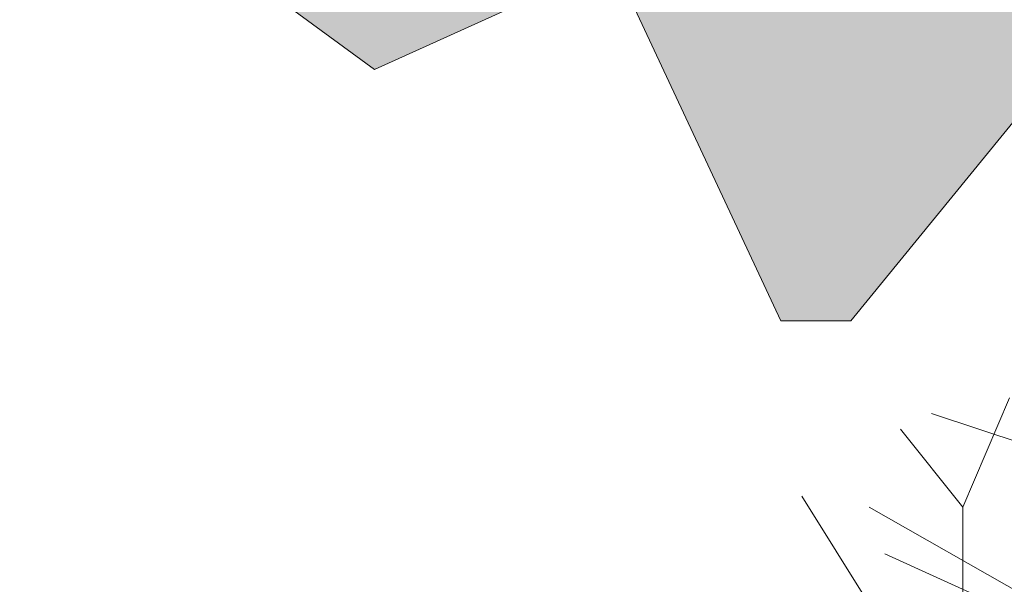
# Model space of a CAD drawing. Units: inches. Extents: x 2091 to 2899, y 967 to 2217.
# Tile 105 of 256: x 2223 to 2254, y 1114 to 1131. Entities that reach past the tile are written whole.
import ezdxf

# ---------------------------------------------------------------- set-up
doc = ezdxf.new("R2010")
doc.units = ezdxf.units.IN
doc.layers.add('A-ANNO-DIMS', color=2, linetype='Continuous', lineweight=18)
doc.layers.add('L-PLNT-TREE', color=94, linetype='Continuous', lineweight=13)
doc.layers.add('A-WALL-PATT', color=141, linetype='Continuous', lineweight=13, true_color=0xadddf7)
doc.layers.add('L-PLNT-PATT', color=114, linetype='Continuous', lineweight=13, true_color=0x139b48)
doc.styles.get("Standard").update_dxf_attribs({"font": 'arial.ttf'})
doc.dimstyles.new('ISO-25', dxfattribs={"dimtxt": 4, "dimasz": 4, "dimexe": 1.25, "dimexo": 0.625, "dimtad": 1, "dimdec": 0, "dimlunit": 3, "dimtxsty": 'Standard', "dimcen": 2.5, "dimadec": 0, "dimazin": 0, "dimtfac": 1, "dimtdec": 0, "dimtmove": 0, "dimatfit": 3, "dimfxl": 1, "dimarcsym": 0})

# ---------------------------------------------------------------- blocks, each defined once
blk = doc.blocks.new('*U25')
blk.add_lwpolyline([(-1139.42368, 1783.79628), (-1216.11644, 1685.47796), (-1117.5111, 1601.2033), (-1051.7759, 1643.3419), (-1126.09884, 1521.20092), (-1072.10606, 1527.49758), (-1079.90386, 1416.93646), (-1259.93906, 1179.83508), (-1479.05978, 1165.78888), (-1577.66258, 1109.60662), (-1742.00312, 927.01364), (-1676.26538, 814.64658), (-1270.89408, 828.69278), (-1194.20386, 772.51052), (-1007.95074, 856.78518), (-876.4778, 575.87134), (-821.70016, 575.87134), (-569.71184, 884.87504)])
blk = doc.blocks.new('*U29')
for p, q in [((-426.72, 414.528), (-390.144, 499.872)), ((-377.952, 463.296), (-451.104, 487.68)), ((-426.72, 414.528), (-475.488, 475.488)), ((-463.296, 280.416), (-552.577, 423.037)), ((-329.184, 316.992), (-499.872, 414.528)), ((-426.72, 316.992), (-426.72, 414.528)), ((-353.568, 316.992), (-487.68, 377.952))]:
    blk.add_line(p, q)
blk = doc.blocks.new('*D71')
at = {"layer": 'A-ANNO-DIMS', "color": 0, "lineweight": -2, "transparency": 16777216}
for p, q in [((2212.144, 1351.294), (2212.144, 969.464)), ((2452.144, 1351.294), (2452.144, 969.464)), ((2216.144, 970.714), (2448.144, 970.714))]:
    blk.add_line(p, q, dxfattribs=at)
at = {"layer": 'A-ANNO-DIMS', "color": 0, "transparency": 16777216}
for points in [[(2216.144, 971.381), (2216.144, 970.048), (2212.144, 970.714)], [(2448.144, 971.381), (2448.144, 970.048), (2452.144, 970.714)]]:
    blk.add_solid(points, dxfattribs=at)
at = {"layer": 'Defpoints', "color": 0, "transparency": 16777216}
for p in [(2212.144, 1351.919), (2452.144, 1351.919), (2452.144, 970.714)]:
    blk.add_point(p, dxfattribs=at)
at = {"layer": 'A-ANNO-DIMS', "color": 0, "transparency": 16777216, "insert": (2332.144, 973.382), "char_height": 4, "attachment_point": 5}
blk.add_mtext('20\'-0"', dxfattribs=at)
blk = doc.blocks.new('*D75')
at = {"layer": 'A-ANNO-DIMS', "color": 0, "lineweight": -2, "transparency": 16777216}
for p, q in [((2212.144, 1274.794), (2212.144, 969.464)), ((2308.144, 1274.794), (2308.144, 969.464)), ((2216.144, 970.714), (2304.144, 970.714))]:
    blk.add_line(p, q, dxfattribs=at)
at = {"layer": 'A-ANNO-DIMS', "color": 0, "transparency": 16777216}
for points in [[(2216.144, 971.381), (2216.144, 970.048), (2212.144, 970.714)], [(2304.144, 971.381), (2304.144, 970.048), (2308.144, 970.714)]]:
    blk.add_solid(points, dxfattribs=at)
at = {"layer": 'Defpoints', "color": 0, "transparency": 16777216}
for p in [(2212.144, 1275.419), (2308.144, 1275.419), (2308.144, 970.714)]:
    blk.add_point(p, dxfattribs=at)
at = {"layer": 'A-ANNO-DIMS', "color": 0, "transparency": 16777216, "insert": (2260.144, 973.382), "char_height": 4, "attachment_point": 5}
blk.add_mtext('8\'-0"', dxfattribs=at)

msp = doc.modelspace()

# ---------------------------------------------------------------- hatches: boundary and pattern name
at = {"layer": 'A-WALL-PATT'}
h = msp.add_hatch(color=256, dxfattribs=at)
h.dxf.hatch_style = 1
h.paths.add_polyline_path([(2803.144, 2050.919), (2203.144, 2050.919), (2203.144, 1090.919), (2803.144, 1090.919)])
h.paths.add_polyline_path([(2635.799, 1147.54), (2674.524, 1147.54, 0.376086), (2678.53, 1152.88), (2678.53, 1159.556, 0.333335), (2674.524, 1163.562), (2674.524, 1163.562), (2674.524, 1192.934), (2635.806, 1192.934), (2597.088, 1192.934), (2597.088, 1163.562, 0.333335), (2593.082, 1159.556), (2593.082, 1152.88, 0.376086), (2597.088, 1147.54)], flags=0)
h.paths.add_polyline_path([(2436.01, 1278.241, 0.000483), (2435.953, 1278.215, -0.001328), (2435.936, 1278.112, -0.001711), (2436.116, 1278.041, 0.002185)], flags=0)
h.paths.add_polyline_path([(2794.144, 1143.419), (2794.144, 1347.419), (2543.37, 1347.419), (2543.37, 1351.919), (2794.144, 1351.919), (2794.144, 1392.714), (2793.947, 1392.714), (2793.947, 1473.537), (2794.144, 1473.537), (2794.144, 1531.919), (2650.144, 1531.919), (2650.144, 1536.419), (2794.144, 1536.419), (2794.144, 1692.419), (2609.376, 1692.419), (2609.376, 1644.419), (2604.876, 1644.419), (2604.876, 1744.919), (2609.376, 1744.919), (2609.376, 1696.919), (2794.144, 1696.919), (2794.144, 1780.919), (2609.644, 1780.919), (2493.876, 1780.919), (2493.876, 1785.419), (2609.644, 1785.419), (2794.144, 1785.419), (2794.144, 1847.939), (2793.951, 1847.939), (2793.951, 1928.762), (2794.144, 1928.762), (2794.144, 1941.419), (2614.144, 1941.419), (2614.144, 1821.419), (2609.644, 1821.419), (2609.644, 1941.419), (2392.144, 1941.419), (2392.144, 1819.919), (2387.644, 1819.919), (2387.644, 1941.419), (2212.144, 1941.419), (2212.144, 1783.919), (2392.144, 1783.919), (2392.144, 1780.919), (2212.144, 1780.919), (2212.144, 1629.419), (2387.644, 1629.419), (2387.644, 1744.919), (2392.144, 1744.919), (2392.144, 1627.919), (2317.144, 1627.919), (2317.144, 1551.419), (2317.144, 1536.419), (2459.384, 1536.419), (2459.384, 1602.396), (2463.884, 1602.396), (2463.884, 1531.919), (2456.644, 1531.919), (2456.644, 1529.919), (2452.144, 1529.919), (2452.144, 1531.919), (2312.644, 1531.919), (2312.644, 1551.419), (2306.144, 1551.419), (2306.144, 1555.919), (2308.144, 1555.919), (2308.144, 1551.419), (2312.644, 1551.419), (2312.644, 1627.919), (2212.144, 1627.919), (2212.144, 1555.919), (2270.144, 1555.919), (2270.144, 1551.419), (2212.144, 1551.419), (2212.144, 1351.919), (2272.144, 1351.919), (2272.144, 1347.419), (2212.144, 1347.419), (2212.144, 1275.419), (2308.144, 1275.419), (2308.144, 1351.919), (2452.144, 1351.919), (2452.144, 1493.919), (2456.644, 1493.919), (2456.644, 1347.419), (2312.644, 1347.419), (2312.644, 1270.919), (2212.144, 1270.919), (2212.144, 1099.919), (2281.238, 1099.919), (2282.871, 1110.914), (2282.008, 1116.997), (2278.558, 1121.42), (2268.206, 1128.056), (2272.088, 1128.056), (2273.813, 1131.927), (2279.42, 1134.692), (2285.028, 1135.245), (2287.616, 1137.457), (2288.047, 1138.01), (2289.341, 1140.775), (2291.067, 1139.669), (2292.361, 1135.245), (2295.38, 1136.904), (2296.243, 1135.798), (2297.105, 1133.033), (2300.125, 1138.01), (2303.144, 1138.01), (2304.438, 1135.798), (2303.144, 1133.586), (2306.595, 1134.692), (2307.889, 1133.033), (2310.908, 1135.245), (2313.927, 1134.139), (2315.627, 1132.427), (2308.32, 1117.55), (2290.204, 1109.808), (2288.91, 1103.172), (2289.272, 1099.919), (2434.918, 1099.919), (2431.593, 1124.788), (2429.93, 1169.553), (2430.927, 1240.52), (2435.659, 1238.186), (2437.135, 1196.554), (2438.798, 1143.973), (2442.678, 1111.998), (2446.558, 1099.919), (2794.144, 1099.919), (2794.144, 1138.919), (2548.032, 1138.919), (2548.032, 1143.419), (2548.032, 1148.819), (2546.668, 1148.032), (2528.686, 1179.179, 0.256256), (2512.032, 1148.819), (2512.032, 1143.419), (2512.032, 1138.919), (2507.532, 1138.919), (2507.532, 1143.419), (2507.532, 1148.819, 0.256256), (2490.879, 1179.179), (2472.896, 1148.032), (2471.532, 1148.819), (2471.532, 1143.419), (2467.032, 1143.419), (2467.032, 1269.946, 0.039061), (2460.91, 1273.58), (2467.032, 1273.58), (2467.032, 1286.325, 0.014511), (2465.216, 1286.762), (2467.032, 1287.053), (2467.032, 1323.419), (2471.532, 1323.419), (2471.532, 1148.819), (2489.532, 1179.996), (2490.896, 1179.208), (2490.879, 1179.179, -0.256256), (2507.532, 1148.819), (2507.532, 1143.419), (2512.032, 1143.419), (2512.032, 1148.819, -0.256256), (2528.686, 1179.179), (2528.668, 1179.208), (2530.032, 1179.996), (2548.032, 1148.819), (2548.032, 1143.419)], flags=16)
h.paths.add_polyline_path([(2607.769, 1200.945), (2607.769, 1265.031), (2597.088, 1281.052), (2619.785, 1281.052), (2627.795, 1337.127), (2635.799, 1337.127), (2643.817, 1337.127), (2651.827, 1281.052), (2674.524, 1281.052), (2663.843, 1265.031), (2663.843, 1200.945), (2635.806, 1200.945)], flags=0)
edge = h.paths.add_edge_path(flags=0)
edge.add_ellipse((13303.896, 1272.999), major_axis=(-10595.313, 0), ratio=0.84230387, start_angle=0.6282372, end_angle=0.6465541, ccw=False)
edge.add_ellipse((2711.7, 1156.853), major_axis=(2.22, 0), ratio=0.842304, start_angle=111.5352, end_angle=180.6282, ccw=False)
edge.add_ellipse((13303.156, 1272.999), major_axis=(-10593.026, 0), ratio=0.84230387, start_angle=0.5282715, end_angle=0.6465541, ccw=False)
edge.add_line((2710.765, 1175.333), (2710.13, 1175.333))
edge.add_ellipse((2710.13, 1176.58), major_axis=(1.48, 0), ratio=0.842304, start_angle=180, end_angle=270, ccw=False)
edge.add_line((2708.65, 1176.58), (2708.65, 1200.783))
edge.add_ellipse((2710.13, 1200.783), major_axis=(1.48, 0), ratio=0.842304, start_angle=90, end_angle=180, ccw=False)
edge.add_line((2710.13, 1202.029), (2710.465, 1202.029))
edge.add_ellipse((13303.156, 1272.999), major_axis=(-10593.026, 0), ratio=0.84230387, start_angle=-0.0902291, end_angle=0.3838668, ccw=False)
edge.add_ellipse((2710.13, 1290.927), major_axis=(-1.48, 0), ratio=0.842304, start_angle=0, end_angle=90, ccw=False)
edge.add_line((2708.65, 1290.927), (2708.65, 1315.13))
edge.add_ellipse((2710.13, 1315.13), major_axis=(-1.48, 0), ratio=0.842304, start_angle=-90, end_angle=0, ccw=False)
edge.add_line((2710.13, 1316.377), (2710.706, 1316.377))
edge.add_ellipse((3238.402, 1296.29), major_axis=(528.234, 0), ratio=0.8423039, start_angle=176.34957, end_angle=177.82005, ccw=False)
edge.add_ellipse((2775.063, 1071.451), major_axis=(313.308, 0), ratio=0.8423039, start_angle=102.12597, end_angle=103.78053, ccw=False)
edge.add_ellipse((2775.063, 1078.306), major_axis=(-305.303, 0), ratio=0.8423039, start_angle=-79.79046, end_angle=-77.55537, ccw=False)
edge.add_ellipse((2695.142, 1541.975), major_axis=(-250.96, 0), ratio=0.8423039, start_angle=99.25657, end_angle=102.55493)
edge.add_line((2741.41, 1334.214), (2747.133, 1337.378))
edge.add_ellipse((2747.539, 1336.857), major_axis=(-0.74, 0), ratio=0.842304, start_angle=270, end_angle=307.9331, ccw=False)
edge.add_ellipse((2747.539, 1336.857), major_axis=(-0.74, 0), ratio=0.842304, start_angle=232.0669, end_angle=270, ccw=False)
edge.add_line((2747.945, 1337.378), (2753.667, 1334.214))
edge.add_ellipse((2799.935, 1541.975), major_axis=(250.96, 0), ratio=0.8423039, start_angle=257.44507, end_angle=260.74343)
edge.add_ellipse((2720.014, 1078.306), major_axis=(305.303, 0), ratio=0.8423039, start_angle=77.55537, end_angle=79.79046, ccw=False)
edge.add_ellipse((2720.014, 1071.451), major_axis=(-313.308, 0), ratio=0.8423039, start_angle=256.21947, end_angle=257.87403, ccw=False)
edge.add_ellipse((2256.676, 1296.29), major_axis=(-528.234, 0), ratio=0.8423039, start_angle=182.17995, end_angle=183.65043, ccw=False)
edge.add_line((2784.371, 1316.377), (2784.947, 1316.377))
edge.add_ellipse((2784.947, 1315.13), major_axis=(1.48, 0), ratio=0.842304, start_angle=0, end_angle=90, ccw=False)
edge.add_line((2786.427, 1315.13), (2786.427, 1290.927))
edge.add_ellipse((2784.947, 1290.927), major_axis=(1.48, 0), ratio=0.842304, start_angle=270, end_angle=360, ccw=False)
edge.add_ellipse((-7808.079, 1272.999), major_axis=(10593.026, 0), ratio=0.84230387, start_angle=-0.3838668, end_angle=0.0902291, ccw=False)
edge.add_line((2784.612, 1202.029), (2784.947, 1202.029))
edge.add_ellipse((2784.947, 1200.783), major_axis=(1.48, 0), ratio=0.842304, start_angle=0, end_angle=90, ccw=False)
edge.add_line((2786.427, 1200.783), (2786.427, 1176.58))
edge.add_ellipse((2784.947, 1176.58), major_axis=(-1.48, 0), ratio=0.842304, start_angle=90, end_angle=180, ccw=False)
edge.add_line((2784.947, 1175.333), (2784.313, 1175.333))
edge.add_ellipse((-7808.079, 1272.999), major_axis=(10593.026, 0), ratio=0.84230387, start_angle=-0.6186432, end_angle=-0.5282715, ccw=False)
edge.add_ellipse((2783.377, 1156.853), major_axis=(-2.22, 0), ratio=0.842304, start_angle=179.3718, end_angle=248.4648, ccw=False)
edge.add_ellipse((-7808.819, 1272.999), major_axis=(-10595.313, 0), ratio=0.842303866, start_angle=179.3534459, end_angle=179.3717628, ccw=False)
edge.add_ellipse((2780.297, 1153.501), major_axis=(-5.246, 0), ratio=0.842304, start_angle=90, end_angle=179.3534, ccw=False)
edge.add_line((2780.297, 1149.082), (2714.78, 1149.082))
edge.add_ellipse((2714.78, 1153.501), major_axis=(5.246, 0), ratio=0.842304, start_angle=180.6466, end_angle=270, ccw=False)
edge = h.paths.add_edge_path(flags=0)
edge.add_line((2718.187, 1151.008), (2718.187, 1170.472))
edge.add_ellipse((2721.147, 1170.472), major_axis=(-2.96, 0), ratio=0.842304, start_angle=-90, end_angle=0, ccw=False)
edge.add_line((2721.147, 1172.965), (2773.93, 1172.965))
edge.add_ellipse((2773.93, 1170.472), major_axis=(-2.96, 0), ratio=0.842304, start_angle=180, end_angle=270, ccw=False)
edge.add_line((2776.89, 1170.472), (2776.89, 1151.008))
edge.add_line((2776.89, 1151.008), (2718.187, 1151.008))
edge = h.paths.add_edge_path(flags=0)
edge.add_line((2718.187, 1180.234), (2718.187, 1199.058))
edge.add_ellipse((2747.539, 1320.399), major_axis=(147.018, 0), ratio=0.8423039, start_angle=256.40187, end_angle=283.59813)
edge.add_line((2776.89, 1199.058), (2776.89, 1180.234))
edge.add_ellipse((2747.539, 1301.575), major_axis=(147.018, 0), ratio=0.8423039, start_angle=256.40187, end_angle=283.59813, ccw=False)
edge = h.paths.add_edge_path(flags=0)
edge.add_ellipse((13303.156, 1272.999), major_axis=(-10591.546, 0), ratio=0.84230387, start_angle=0.0555943, end_angle=0.3777642, ccw=False)
edge.add_line((2711.617, 1262.722), (2715.667, 1249.495))
edge.add_ellipse((6413.892, 1241.692), major_axis=(-3698.236, 0), ratio=0.84230387, start_angle=-0.120897, end_angle=0.364076)
edge.add_line((2715.761, 1218.192), (2711.934, 1203.167))
edge = h.paths.add_edge_path(flags=0)
edge.add_line((2718.187, 1251.075), (2716.002, 1267.45))
edge.add_ellipse((2742.151, 1202.19), major_axis=(81.773, 0), ratio=0.842304, start_angle=94.27742, end_angle=111.83495, ccw=False)
edge.add_line((2737.01, 1270.931), (2758.067, 1270.931))
edge.add_ellipse((2752.926, 1202.19), major_axis=(81.773, 0), ratio=0.842304, start_angle=68.16505, end_angle=85.72258, ccw=False)
edge.add_line((2779.075, 1267.45), (2776.89, 1251.075))
edge.add_ellipse((2750.338, 1187.885), major_axis=(79.58, 0), ratio=0.842304, start_angle=67.20809, end_angle=85.12993)
edge.add_line((2756.035, 1254.744), (2739.043, 1254.744))
edge.add_ellipse((2744.739, 1187.885), major_axis=(79.58, 0), ratio=0.842304, start_angle=94.87007, end_angle=112.79191)
edge = h.paths.add_edge_path(flags=0)
edge.add_line((2783.143, 1203.167), (2779.316, 1218.192))
edge.add_ellipse((-918.815, 1241.692), major_axis=(3698.236, 0), ratio=0.84230387, start_angle=-0.364076, end_angle=0.120897)
edge.add_line((2779.41, 1249.495), (2783.46, 1262.722))
edge.add_ellipse((-7808.079, 1272.999), major_axis=(-10591.546, 0), ratio=0.84230387, start_angle=179.6222358, end_angle=179.9444057, ccw=False)
edge = h.paths.add_edge_path(flags=0)
edge.add_ellipse((2734.201, 1286.69), major_axis=(-0.357, 6.34), ratio=0.603834, start_angle=89.002, end_angle=253.6574, ccw=False)
edge.add_line((2730.369, 1286.542), (2730.369, 1301.352))
edge.add_line((2730.369, 1301.352), (2735.913, 1305.215))
edge.add_ellipse((2736.385, 1304.735), major_axis=(0.74, 0), ratio=0.842304, start_angle=90, end_angle=134.4802, ccw=False)
edge.add_line((2736.385, 1305.358), (2738.033, 1305.358))
edge.add_line((2738.033, 1305.358), (2738.033, 1307.708))
edge.add_ellipse((2794.202, 1307.708), major_axis=(56.169, 0), ratio=0.842304, start_angle=150.5614, end_angle=180, ccw=False)
edge.add_ellipse((2700.876, 1307.708), major_axis=(-56.169, 0), ratio=0.842304, start_angle=180, end_angle=209.4386, ccw=False)
edge.add_line((2757.044, 1307.708), (2757.044, 1305.358))
edge.add_line((2757.044, 1305.358), (2758.692, 1305.358))
edge.add_ellipse((2758.692, 1304.735), major_axis=(-0.74, 0), ratio=0.842304, start_angle=225.5198, end_angle=270, ccw=False)
edge.add_line((2759.164, 1305.215), (2764.708, 1301.352))
edge.add_line((2764.708, 1301.352), (2764.708, 1286.542))
edge.add_ellipse((2760.876, 1286.69), major_axis=(0.357, 6.34), ratio=0.603834, start_angle=106.3426, end_angle=270.998, ccw=False)
edge.add_line((2757.044, 1285.797), (2757.044, 1307.708))
edge.add_ellipse((2700.876, 1307.708), major_axis=(-56.169, 0), ratio=0.842304, start_angle=180, end_angle=209.4386)
edge.add_ellipse((2794.202, 1307.708), major_axis=(56.169, 0), ratio=0.842304, start_angle=150.5614, end_angle=180)
edge.add_line((2738.033, 1307.708), (2738.033, 1285.797))
h.paths.add_polyline_path([(2417.812, 1104.45), (2413.492, 1102.53), (2410.612, 1103.97), (2409.172, 1106.37), (2407.252, 1107.33), (2406.292, 1109.73), (2405.332, 1114.05), (2405.332, 1117.89), (2406.292, 1120.13), (2407.252, 1119.81), (2408.848, 1118.328), (2410.174, 1119.424), (2410.211, 1120.406), (2411.041, 1121.419), (2410.699, 1119.859), (2410.174, 1119.424), (2410.088, 1117.176), (2411.133, 1116.206), (2413.972, 1119.33), (2416.852, 1120.77), (2416.87, 1120.799), (2417.035, 1119.405), (2417.896, 1118.143), (2418.292, 1118.37), (2419.544, 1120.039), (2419.361, 1118.387), (2419.032, 1119.356), (2418.399, 1118.512), (2419.252, 1114.53), (2418.794, 1107.199)], flags=0)
h.paths.add_polyline_path([(2508.87, 1347.419), (2508.37, 1347.419), (2508.37, 1351.919), (2508.87, 1351.919)], flags=0)
h.paths.add_polyline_path([(2473.37, 1347.419), (2472.37, 1347.419), (2467.87, 1347.419), (2467.87, 1455.419), (2472.37, 1455.419), (2472.37, 1352.419), (2473.37, 1352.419)], flags=0)
h.paths.add_polyline_path([(2352.106, 1217.446), (2349.226, 1218.886), (2347.786, 1221.286), (2345.866, 1222.246), (2344.906, 1224.646), (2343.946, 1228.966), (2343.946, 1232.806), (2344.906, 1235.046), (2345.866, 1234.726), (2347.462, 1233.244), (2348.788, 1234.341), (2348.825, 1235.322), (2349.655, 1236.336), (2349.313, 1234.775), (2348.788, 1234.341), (2348.702, 1232.093), (2349.747, 1231.123), (2352.586, 1234.246), (2355.466, 1235.686), (2355.484, 1235.715), (2355.649, 1234.322), (2356.51, 1233.06), (2356.906, 1233.286), (2358.158, 1234.956), (2357.975, 1233.304), (2357.646, 1234.273), (2357.013, 1233.428), (2357.866, 1229.446), (2357.408, 1222.115), (2356.426, 1219.366)], flags=0)
h.paths.add_polyline_path([(2348.297, 1112.224), (2347.014, 1112.31), (2345.53, 1114.127), (2345.732, 1115.858), (2346.812, 1116.982), (2346.812, 1114.646), (2345.867, 1114.214), (2346.88, 1114.3)], flags=0)
h.paths.add_polyline_path([(2347.014, 1110.926), (2346.272, 1110.493), (2346.61, 1111.186)], flags=0)
h.paths.add_polyline_path([(2345.867, 1118.194), (2345.53, 1117.329), (2343.708, 1118.021), (2344.383, 1118.626)], flags=0)
h.paths.add_polyline_path([(2346.677, 1109.282), (2346.07, 1108.071), (2345.867, 1110.061)], flags=0)
h.paths.add_polyline_path([(2345.057, 1119.751), (2343.64, 1119.751), (2343.978, 1121.135)], flags=0)
h.paths.add_polyline_path([(2345.26, 1116.55), (2345.125, 1115.858), (2344.922, 1115.685), (2344.72, 1116.377)], flags=0)
h.paths.add_polyline_path([(2345.665, 1112.31), (2345.462, 1111.532), (2344.045, 1111.964), (2344.652, 1112.57)], flags=0)
h.paths.add_polyline_path([(2345.192, 1113.349), (2344.45, 1113.868), (2344.72, 1114.387)], flags=0)
h.paths.add_polyline_path([(2344.652, 1116.809), (2344.18, 1115.685), (2344.652, 1115.339), (2343.91, 1114.906), (2343.033, 1115.944), (2343.64, 1116.463)], flags=0)
h.paths.add_polyline_path([(2345.867, 1106.686), (2344.99, 1105.562), (2344.517, 1106.6)], flags=0)
h.paths.add_polyline_path([(2344.855, 1110.061), (2344.517, 1109.282), (2344.113, 1109.715)], flags=0)
h.paths.add_polyline_path([(2344.045, 1113.522), (2343.438, 1113.089), (2342.763, 1113.954)], flags=0)
h.paths.add_polyline_path([(2344.315, 1111.012), (2342.965, 1110.32), (2342.965, 1111.099)], flags=0)
h.paths.add_polyline_path([(2345.125, 1104.697), (2344.585, 1103.745), (2344.45, 1104.264)], flags=0)
h.paths.add_polyline_path([(2342.83, 1121.222), (2341.75, 1120.53), (2340.536, 1121.049), (2340.131, 1121.828), (2340.671, 1122.952), (2341.143, 1121.828), (2341.615, 1122.001)], flags=0)
h.paths.add_polyline_path([(2342.965, 1119.751), (2343.033, 1118.453), (2342.088, 1118.021), (2342.02, 1119.491)], flags=0)
h.paths.add_polyline_path([(2342.695, 1116.896), (2341.953, 1116.636), (2342.02, 1117.329)], flags=0)
h.paths.add_polyline_path([(2343.033, 1112.224), (2342.02, 1111.791), (2341.548, 1112.224), (2342.358, 1113.349)], flags=0)
h.paths.add_polyline_path([(2343.775, 1104.437), (2342.628, 1102.88), (2342.695, 1104.61), (2343.438, 1105.129)], flags=0)
h.paths.add_polyline_path([(2342.02, 1115.079), (2340.806, 1115.512), (2340.941, 1116.377)], flags=0)
h.paths.add_polyline_path([(2341.481, 1120.097), (2341.481, 1119.405), (2341.076, 1119.578), (2341.143, 1120.097)], flags=0)
h.paths.add_polyline_path([(2341.818, 1114.473), (2340.941, 1113.089), (2340.806, 1114.56)], flags=0)
h.paths.add_polyline_path([(2341.143, 1118.54), (2340.941, 1116.982), (2339.051, 1117.675), (2339.051, 1118.626)], flags=0)
h.paths.add_polyline_path([(2342.695, 1101.668), (2341.953, 1101.841), (2342.56, 1102.361)], flags=0)
h.paths.add_polyline_path([(2340.333, 1119.665), (2338.444, 1119.578), (2337.904, 1120.357), (2339.658, 1120.616)], flags=0)
h.paths.add_polyline_path([(2340.333, 1115.339), (2340.063, 1113.695), (2339.388, 1115.339)], flags=0)
h.paths.add_polyline_path([(2341.818, 1103.831), (2341.548, 1102.88), (2341.143, 1103.658)], flags=0)
h.paths.add_polyline_path([(2339.051, 1122.866), (2337.296, 1121.828), (2337.094, 1123.125), (2337.769, 1123.818)], flags=0)
h.paths.add_polyline_path([(2339.118, 1121.741), (2338.848, 1121.222), (2338.174, 1121.049), (2338.376, 1121.568)], flags=0)
h.paths.add_polyline_path([(2339.186, 1119.319), (2338.646, 1118.713), (2338.241, 1118.107), (2338.241, 1118.886)], flags=0)
h.paths.add_polyline_path([(2341.143, 1101.928), (2340.603, 1101.236), (2340.063, 1101.841), (2340.603, 1102.361)], flags=0)
h.paths.add_polyline_path([(2337.634, 1117.761), (2336.621, 1118.28), (2337.296, 1118.972)], flags=0)
h.paths.add_polyline_path([(2336.824, 1119.578), (2334.799, 1118.972), (2335.204, 1120.357), (2336.554, 1120.876)], flags=0)
h.paths.add_polyline_path([(2339.118, 1100.457), (2337.364, 1100.543), (2336.756, 1101.236)], flags=0)
h.paths.add_polyline_path([(2336.351, 1122.433), (2336.014, 1121.914), (2334.934, 1122.433), (2334.529, 1123.471), (2335.744, 1122.779)], flags=0)
h.paths.add_polyline_path([(2334.732, 1120.876), (2334.259, 1120.357), (2334.057, 1120.789), (2334.597, 1121.308)], flags=0)
h.paths.add_polyline_path([(2334.462, 1122.174), (2332.572, 1121.308), (2331.357, 1122.174), (2332.1, 1122.866)], flags=0)
h.paths.add_polyline_path([(2334.259, 1118.54), (2333.382, 1118.453), (2333.652, 1119.319)], flags=0)
h.paths.add_polyline_path([(2335.542, 1102.274), (2334.192, 1102.62), (2335.272, 1103.312)], flags=0)
h.paths.add_polyline_path([(2332.707, 1119.665), (2331.695, 1120.443), (2332.505, 1120.789)], flags=0)
h.paths.add_polyline_path([(2334.732, 1101.149), (2333.517, 1101.582), (2333.989, 1101.755)], flags=0)
h.paths.add_polyline_path([(2332.64, 1116.636), (2331.087, 1116.29), (2331.965, 1118.194)], flags=0)
h.paths.add_polyline_path([(2330.75, 1121.568), (2330.277, 1120.27), (2328.523, 1119.319), (2328.995, 1121.049)], flags=0)
h.paths.add_polyline_path([(2330.75, 1118.626), (2330.008, 1117.502), (2329.873, 1118.021)], flags=0)
h.paths.add_polyline_path([(2332.1, 1102.361), (2330.547, 1102.014), (2331.695, 1102.966)], flags=0)
h.paths.add_polyline_path([(2329.535, 1113.608), (2329.063, 1112.31), (2328.59, 1113.349)], flags=0)
h.paths.add_polyline_path([(2328.388, 1117.848), (2327.51, 1116.55), (2327.173, 1117.761)], flags=0)
h.paths.add_polyline_path([(2329.738, 1106.513), (2329.535, 1105.302), (2328.253, 1106.081)], flags=0)
h.paths.add_polyline_path([(2328.658, 1114.387), (2328.05, 1114.127), (2328.32, 1114.906)], flags=0)
h.paths.add_polyline_path([(2328.32, 1112.224), (2327.106, 1112.137), (2326.701, 1112.656)], flags=0)
h.paths.add_polyline_path([(2326.903, 1115.252), (2326.701, 1114.127), (2325.216, 1113.608), (2326.093, 1115.339)], flags=0)
h.paths.add_polyline_path([(2326.633, 1108.33), (2326.093, 1107.379), (2325.891, 1108.503), (2326.498, 1109.109)], flags=0)
h.paths.add_polyline_path([(2615.144, 1531.919), (2609.644, 1531.919), (2609.644, 1620.419), (2614.144, 1620.419), (2614.144, 1536.419), (2615.144, 1536.419)], flags=0)
h.paths.add_polyline_path([(2545.144, 1563.419), (2464.144, 1563.419), (2464.144, 1632.419), (2509.144, 1632.419), (2509.144, 1627.919), (2509.144, 1603.919), (2468.644, 1603.919), (2468.644, 1567.919), (2540.644, 1567.919), (2540.644, 1591.919), (2545.144, 1591.919)], flags=0)
h.paths.add_polyline_path([(2388.969, 1549.986), (2357.434, 1549.986), (2357.434, 1623.361), (2399.363, 1623.361), (2435.689, 1623.361), (2435.593, 1602.559), (2435.593, 1602.396), (2388.969, 1602.396)], flags=0)
h.paths.add_polyline_path([(2388.881, 1555.809), (2374.904, 1555.809), (2374.904, 1600.572), (2374.904, 1615.458), (2406.351, 1615.458), (2406.351, 1618.939), (2412.174, 1615.458), (2406.351, 1611.976), (2406.351, 1615.458), (2388.881, 1615.458)], flags=0)
h.paths.add_polyline_path([(2568.876, 1644.419), (2453.376, 1644.419), (2453.376, 1785.419), (2457.876, 1785.419), (2457.876, 1648.919), (2568.876, 1648.919)], flags=0)
h.paths.add_polyline_path([(2212.144, 1945.919), (2212.144, 2041.919), (2794.144, 2041.919), (2794.144, 1945.919)], flags=16)
h.paths.add_polyline_path([(2271.083, 1964.317), (2776.853, 1964.317), (2776.853, 2037.17), (2271.083, 2037.17)], flags=8)
h.paths.add_polyline_path([(2380.649, 1536.824), (2461.041, 1536.824), (2461.041, 1554.653), (2380.649, 1554.653)], flags=8)
h.paths.add_polyline_path([(2240.756, 1609.725), (2309.186, 1609.725), (2309.186, 1617.698), (2240.756, 1617.698)], flags=8)
h.paths.add_polyline_path([(2212.677, 1313.504), (2282.592, 1313.504), (2282.592, 1322.745), (2212.677, 1322.745)], flags=8)
h.paths.add_polyline_path([(2457.112, 1114.779), (2558.482, 1114.779), (2558.482, 1142.22), (2457.112, 1142.22)], flags=8)
h.paths.add_polyline_path([(2473.442, 1273.01), (2604.641, 1273.01), (2604.641, 1318.347), (2473.442, 1318.347)], flags=8)
h.paths.add_polyline_path([(2638.876, 1626.977), (2684.25, 1627.977), (2684.038, 1637.597), (2638.664, 1636.598)], flags=8)
h.paths.add_polyline_path([(2537.591, 1453.793), (2628.39, 1453.793), (2628.39, 1475.345), (2537.591, 1475.345)], flags=8)
h.paths.add_polyline_path([(2504.138, 1714.632), (2554.647, 1714.632), (2554.647, 1730.238), (2504.138, 1730.238)], flags=8)
h.paths.add_polyline_path([(2487.501, 1575.652), (2535.097, 1575.652), (2535.097, 1598.378), (2487.501, 1598.378)], flags=8)
h.paths.add_polyline_path([(2709.099, 1735.71), (2740.017, 1735.71), (2740.017, 1749.938), (2709.099, 1749.938)], flags=8)
h.paths.add_polyline_path([(2442.438, 1792.172), (2564.729, 1792.172), (2564.729, 1842), (2442.438, 1842)], flags=8)
h.paths.add_polyline_path([(2655.816, 1809.644), (2789.52, 1806.694), (2790.085, 1832.292), (2656.381, 1835.242)], flags=8)
h.paths.add_polyline_path([(2234.843, 1797.72), (2368.593, 1794.769), (2369.161, 1820.504), (2235.411, 1823.455)], flags=8)
h.paths.add_polyline_path([(2245.138, 1644.006), (2398.428, 1640.624), (2398.995, 1666.325), (2245.706, 1669.707)], flags=8)
h.paths.add_polyline_path([(2306.143, 1431.169), (2413.768, 1428.794), (2414.333, 1454.392), (2306.708, 1456.766)], flags=8)
h.paths.add_polyline_path([(2306.835, 1458.233), (2393.38, 1456.323), (2393.933, 1481.354), (2307.387, 1483.264)], flags=8)
at = {"layer": 'L-PLNT-PATT'}
h = msp.add_hatch(color=256, dxfattribs=at)
h.dxf.hatch_style = 1
h.paths.add_polyline_path([(2333.338, 1165.659), (2329.024, 1166.212), (2331.612, 1168.424), (2335.063, 1177.271), (2328.162, 1184.46), (2319.535, 1187.225), (2323.417, 1193.308), (2319.966, 1203.814), (2317.809, 1203.814), (2313.496, 1213.215), (2310.908, 1212.662), (2307.889, 1212.662), (2305.732, 1217.086), (2307.026, 1223.168), (2310.477, 1223.168), (2304.007, 1230.91), (2303.136, 1237.046), (2299.693, 1240.864), (2296.674, 1237.546), (2294.949, 1238.652), (2294.517, 1241.417), (2292.361, 1242.523), (2289.341, 1239.758), (2285.89, 1240.311), (2283.302, 1235.334), (2283.302, 1230.91), (2286.753, 1229.251), (2284.165, 1227.592), (2281.577, 1229.804), (2274.244, 1222.615), (2274.244, 1220.957), (2271.225, 1219.298), (2272.088, 1217.639), (2274.244, 1214.321), (2270.362, 1211.556), (2266.48, 1214.321), (2264.324, 1213.768), (2263.461, 1211.556), (2266.48, 1211.003), (2266.912, 1206.579), (2263.539, 1207.132), (2259.579, 1203.261), (2263.892, 1202.708), (2262.167, 1197.178), (2258.285, 1196.625), (2253.971, 1193.861), (2248.795, 1191.096), (2248.364, 1193.308), (2244.482, 1185.013), (2251.383, 1186.672), (2255.697, 1183.907), (2254.403, 1177.271), (2246.639, 1174.506), (2243.188, 1176.718), (2241.894, 1173.4), (2238.875, 1172.847), (2236.287, 1169.53), (2233.267, 1165.659), (2237.149, 1162.341), (2239.737, 1164), (2236.811, 1159.191), (2238.937, 1159.439), (2238.63, 1155.086), (2231.542, 1145.752), (2222.915, 1145.199), (2219.033, 1142.987), (2212.563, 1135.798), (2215.151, 1131.374), (2231.111, 1131.927), (2234.13, 1129.715), (2241.463, 1133.033), (2246.639, 1121.973), (2248.795, 1121.973), (2258.716, 1134.139), (2261.736, 1135.798), (2263.892, 1133.033), (2263.892, 1129.162), (2267.343, 1128.056), (2272.088, 1128.056), (2273.813, 1131.927), (2279.42, 1134.692), (2285.028, 1135.245), (2287.616, 1137.457), (2288.047, 1138.01), (2289.341, 1140.775), (2291.067, 1139.669), (2292.361, 1135.245), (2295.38, 1136.904), (2296.243, 1135.798), (2297.105, 1133.033), (2300.125, 1138.01), (2303.144, 1138.01), (2304.438, 1135.798), (2303.144, 1133.586), (2306.595, 1134.692), (2307.889, 1133.033), (2310.908, 1135.245), (2313.927, 1134.139), (2319.966, 1128.056), (2322.554, 1126.95), (2324.711, 1124.738), (2342.827, 1126.397), (2346.278, 1123.079), (2348.866, 1124.185), (2341.964, 1133.033), (2341.533, 1136.351), (2343.69, 1139.669), (2339.808, 1150.175), (2337.651, 1150.175)])
h.paths.add_polyline_path([(2339.658, 1120.616), (2337.904, 1120.357), (2338.444, 1119.578), (2340.333, 1119.665)])
h.paths.add_polyline_path([(2341.143, 1118.54), (2339.051, 1118.626), (2339.051, 1117.675), (2340.941, 1116.982)])
h.paths.add_polyline_path([(2336.554, 1120.876), (2335.204, 1120.357), (2334.799, 1118.972), (2336.824, 1119.578)])
h.paths.add_polyline_path([(2337.296, 1118.972), (2336.621, 1118.28), (2337.634, 1117.761)])
h.paths.add_polyline_path([(2338.646, 1118.713), (2339.186, 1119.319), (2338.241, 1118.886), (2338.241, 1118.107)])
h.paths.add_polyline_path([(2339.051, 1122.866), (2337.769, 1123.818), (2337.094, 1123.125), (2337.296, 1121.828)])
h.paths.add_polyline_path([(2341.615, 1122.001), (2341.143, 1121.828), (2340.671, 1122.952), (2340.131, 1121.828), (2340.536, 1121.049), (2341.75, 1120.53), (2342.83, 1121.222)])
h.paths.add_polyline_path([(2342.965, 1119.751), (2342.02, 1119.491), (2342.088, 1118.021), (2343.033, 1118.453)])
h.paths.add_polyline_path([(2345.867, 1118.194), (2344.383, 1118.626), (2343.708, 1118.021), (2345.53, 1117.329)])
h.paths.add_polyline_path([(2344.652, 1116.809), (2343.64, 1116.463), (2343.033, 1115.944), (2343.91, 1114.906), (2344.652, 1115.339), (2344.18, 1115.685)])
h.paths.add_polyline_path([(2346.812, 1116.982), (2345.732, 1115.858), (2345.53, 1114.127), (2347.014, 1112.31), (2348.297, 1112.224), (2346.88, 1114.3), (2345.867, 1114.214), (2346.812, 1114.646)])
h.paths.add_polyline_path([(2345.26, 1116.55), (2344.72, 1116.377), (2344.922, 1115.685), (2345.125, 1115.858)])
h.paths.add_polyline_path([(2342.695, 1116.896), (2342.02, 1117.329), (2341.953, 1116.636)])
h.paths.add_polyline_path([(2341.481, 1120.097), (2341.143, 1120.097), (2341.076, 1119.578), (2341.481, 1119.405)])
h.paths.add_polyline_path([(2343.978, 1121.135), (2343.64, 1119.751), (2345.057, 1119.751)])
h.paths.add_polyline_path([(2339.118, 1121.741), (2338.376, 1121.568), (2338.174, 1121.049), (2338.848, 1121.222)])
h.paths.add_polyline_path([(2336.351, 1122.433), (2335.744, 1122.779), (2334.529, 1123.471), (2334.934, 1122.433), (2336.014, 1121.914)])
h.paths.add_polyline_path([(2334.462, 1122.174), (2332.1, 1122.866), (2331.357, 1122.174), (2332.572, 1121.308)])
h.paths.add_polyline_path([(2334.597, 1121.308), (2334.057, 1120.789), (2334.259, 1120.357), (2334.732, 1120.876)])
h.paths.add_polyline_path([(2332.505, 1120.789), (2331.695, 1120.443), (2332.707, 1119.665)])
h.paths.add_polyline_path([(2333.652, 1119.319), (2333.382, 1118.453), (2334.259, 1118.54)])
h.paths.add_polyline_path([(2331.965, 1118.194), (2331.087, 1116.29), (2332.64, 1116.636)])
h.paths.add_polyline_path([(2330.75, 1121.568), (2328.995, 1121.049), (2328.523, 1119.319), (2330.277, 1120.27)])
h.paths.add_polyline_path([(2330.75, 1118.626), (2329.873, 1118.021), (2330.008, 1117.502)])
h.paths.add_polyline_path([(2328.388, 1117.848), (2327.173, 1117.761), (2327.51, 1116.55)])
h.paths.add_polyline_path([(2326.903, 1115.252), (2326.093, 1115.339), (2325.216, 1113.608), (2326.701, 1114.127)])
h.paths.add_polyline_path([(2328.658, 1114.387), (2328.32, 1114.906), (2328.05, 1114.127)])
h.paths.add_polyline_path([(2326.701, 1112.656), (2327.106, 1112.137), (2328.32, 1112.224)])
h.paths.add_polyline_path([(2329.535, 1113.608), (2328.59, 1113.349), (2329.063, 1112.31)])
h.paths.add_polyline_path([(2340.333, 1115.339), (2339.388, 1115.339), (2340.063, 1113.695)])
h.paths.add_polyline_path([(2340.941, 1116.377), (2340.806, 1115.512), (2342.02, 1115.079)])
h.paths.add_polyline_path([(2341.818, 1114.473), (2340.806, 1114.56), (2340.941, 1113.089)])
h.paths.add_polyline_path([(2343.033, 1112.224), (2342.358, 1113.349), (2341.548, 1112.224), (2342.02, 1111.791)])
h.paths.add_polyline_path([(2342.763, 1113.954), (2343.438, 1113.089), (2344.045, 1113.522)])
h.paths.add_polyline_path([(2344.72, 1114.387), (2344.45, 1113.868), (2345.192, 1113.349)])
h.paths.add_polyline_path([(2345.665, 1112.31), (2344.652, 1112.57), (2344.045, 1111.964), (2345.462, 1111.532)])
h.paths.add_polyline_path([(2344.315, 1111.012), (2342.965, 1111.099), (2342.965, 1110.32)])
h.paths.add_polyline_path([(2344.855, 1110.061), (2344.113, 1109.715), (2344.517, 1109.282)])
h.paths.add_polyline_path([(2346.677, 1109.282), (2345.867, 1110.061), (2346.07, 1108.071)])
h.paths.add_polyline_path([(2347.014, 1110.926), (2346.61, 1111.186), (2346.272, 1110.493)])
h.paths.add_polyline_path([(2345.867, 1106.686), (2344.517, 1106.6), (2344.99, 1105.562)])
h.paths.add_polyline_path([(2345.125, 1104.697), (2344.45, 1104.264), (2344.585, 1103.745)])
h.paths.add_polyline_path([(2343.775, 1104.437), (2343.438, 1105.129), (2342.695, 1104.61), (2342.628, 1102.88)])
h.paths.add_polyline_path([(2341.818, 1103.831), (2341.143, 1103.658), (2341.548, 1102.88)])
h.paths.add_polyline_path([(2342.56, 1102.361), (2341.953, 1101.841), (2342.695, 1101.668)])
h.paths.add_polyline_path([(2341.143, 1101.928), (2340.603, 1102.361), (2340.063, 1101.841), (2340.603, 1101.236)])
h.paths.add_polyline_path([(2336.756, 1101.236), (2337.364, 1100.543), (2339.118, 1100.457)])
h.paths.add_polyline_path([(2335.272, 1103.312), (2334.192, 1102.62), (2335.542, 1102.274)])
h.paths.add_polyline_path([(2333.989, 1101.755), (2333.517, 1101.582), (2334.732, 1101.149)])
h.paths.add_polyline_path([(2331.695, 1102.966), (2330.547, 1102.014), (2332.1, 1102.361)])
h.paths.add_polyline_path([(2329.738, 1106.513), (2328.253, 1106.081), (2329.535, 1105.302)])
h.paths.add_polyline_path([(2326.633, 1108.33), (2326.498, 1109.109), (2325.891, 1108.503), (2326.093, 1107.379)])
h.paths.add_polyline_path([(2240.596, 1257.814), (2239.584, 1257.468), (2238.977, 1256.949), (2239.854, 1255.911), (2240.596, 1256.344), (2240.124, 1256.69)])
h.paths.add_polyline_path([(2241.811, 1259.199), (2240.327, 1259.631), (2239.652, 1259.026), (2241.474, 1258.334)])
h.paths.add_polyline_path([(2242.756, 1257.987), (2241.676, 1256.863), (2241.474, 1255.132), (2242.958, 1253.315), (2244.241, 1253.229), (2242.824, 1255.305), (2241.811, 1255.219), (2242.756, 1255.651)])
h.paths.add_polyline_path([(2241.609, 1253.315), (2240.596, 1253.575), (2239.989, 1252.969), (2241.406, 1252.537)])
h.paths.add_polyline_path([(2240.664, 1255.392), (2240.394, 1254.873), (2241.136, 1254.354)])
h.paths.add_polyline_path([(2242.958, 1251.931), (2242.554, 1252.191), (2242.216, 1251.498)])
h.paths.add_polyline_path([(2240.259, 1252.017), (2238.909, 1252.104), (2238.909, 1251.325)])
h.paths.add_polyline_path([(2238.302, 1254.354), (2237.492, 1253.229), (2237.964, 1252.796), (2238.977, 1253.229)])
h.paths.add_polyline_path([(2239.989, 1254.527), (2238.707, 1254.959), (2239.382, 1254.094)])
h.paths.add_polyline_path([(2240.799, 1251.066), (2240.057, 1250.72), (2240.461, 1250.287)])
h.paths.add_polyline_path([(2241.811, 1251.066), (2242.014, 1249.076), (2242.621, 1250.287)])
h.paths.add_polyline_path([(2241.204, 1257.555), (2240.664, 1257.382), (2240.866, 1256.69), (2241.069, 1256.863)])
h.paths.add_polyline_path([(2238.639, 1257.901), (2237.964, 1258.334), (2237.897, 1257.641)])
h.paths.add_polyline_path([(2238.909, 1260.756), (2237.964, 1260.496), (2238.032, 1259.026), (2238.977, 1259.458)])
h.paths.add_polyline_path([(2239.922, 1262.14), (2239.584, 1260.756), (2241.001, 1260.756)])
h.paths.add_polyline_path([(2238.774, 1262.227), (2237.559, 1263.006), (2237.087, 1262.833), (2236.615, 1263.957), (2236.075, 1262.833), (2236.48, 1262.054), (2237.694, 1261.535)])
h.paths.add_polyline_path([(2237.425, 1261.102), (2237.087, 1261.102), (2237.02, 1260.583), (2237.425, 1260.41)])
h.paths.add_polyline_path([(2237.087, 1259.545), (2234.995, 1259.631), (2234.995, 1258.68), (2236.885, 1257.987)])
h.paths.add_polyline_path([(2236.885, 1257.382), (2236.75, 1256.517), (2237.964, 1256.084)])
h.paths.add_polyline_path([(2237.762, 1255.478), (2236.75, 1255.565), (2236.885, 1254.094)])
h.paths.add_polyline_path([(2236.277, 1256.344), (2235.332, 1256.344), (2236.007, 1254.7)])
h.paths.add_polyline_path([(2241.811, 1247.691), (2240.461, 1247.605), (2240.934, 1246.567)])
h.paths.add_polyline_path([(2239.719, 1245.442), (2239.382, 1246.134), (2238.639, 1245.615), (2238.572, 1243.885)])
h.paths.add_polyline_path([(2241.069, 1245.702), (2240.394, 1245.269), (2240.529, 1244.75)])
h.paths.add_polyline_path([(2237.762, 1244.836), (2237.087, 1244.663), (2237.492, 1243.885)])
h.paths.add_polyline_path([(2237.087, 1242.933), (2236.547, 1243.366), (2236.007, 1242.846), (2236.547, 1242.241)])
h.paths.add_polyline_path([(2238.504, 1243.366), (2237.897, 1242.846), (2238.639, 1242.673)])
h.paths.add_polyline_path([(2232.7, 1242.241), (2233.308, 1241.548), (2235.062, 1241.462)], flags=17)
h.paths.add_polyline_path([(2231.216, 1244.317), (2230.136, 1243.625), (2231.486, 1243.279)])
h.paths.add_polyline_path([(2229.933, 1242.76), (2229.461, 1242.587), (2230.676, 1242.154)])
h.paths.add_polyline_path([(2227.639, 1243.971), (2226.491, 1243.019), (2228.044, 1243.366)])
h.paths.add_polyline_path([(2222.577, 1249.335), (2222.442, 1250.114), (2221.835, 1249.508), (2222.037, 1248.384)])
h.paths.add_polyline_path([(2225.682, 1247.518), (2224.197, 1247.086), (2225.479, 1246.307)])
h.paths.add_polyline_path([(2225.479, 1254.613), (2224.534, 1254.354), (2225.007, 1253.315)])
h.paths.add_polyline_path([(2224.264, 1253.229), (2222.645, 1253.661), (2223.05, 1253.142)])
h.paths.add_polyline_path([(2222.847, 1256.257), (2222.037, 1256.344), (2221.16, 1254.613), (2222.645, 1255.132)])
h.paths.add_polyline_path([(2224.332, 1258.853), (2223.117, 1258.766), (2223.454, 1257.555)])
h.paths.add_polyline_path([(2226.694, 1259.631), (2225.817, 1259.026), (2225.952, 1258.507)])
h.paths.add_polyline_path([(2227.909, 1259.199), (2227.031, 1257.295), (2228.584, 1257.641)])
h.paths.add_polyline_path([(2224.264, 1255.911), (2223.994, 1255.132), (2224.602, 1255.392)])
h.paths.add_polyline_path([(2229.596, 1260.324), (2229.326, 1259.458), (2230.203, 1259.545)])
h.paths.add_polyline_path([(2228.449, 1261.794), (2227.639, 1261.448), (2228.651, 1260.67)])
h.paths.add_polyline_path([(2230.406, 1263.179), (2228.044, 1263.871), (2227.301, 1263.179), (2228.516, 1262.313)])
h.paths.add_polyline_path([(2232.768, 1260.583), (2232.498, 1261.881), (2231.148, 1261.362), (2230.743, 1259.977)])
h.paths.add_polyline_path([(2230.676, 1261.881), (2230.541, 1262.313), (2230.001, 1261.794), (2230.203, 1261.362)])
h.paths.add_polyline_path([(2232.295, 1263.438), (2231.688, 1263.784), (2230.473, 1264.476), (2230.878, 1263.438), (2231.958, 1262.919)])
h.paths.add_polyline_path([(2234.995, 1263.871), (2233.713, 1264.823), (2233.038, 1264.13), (2233.24, 1262.833)])
h.paths.add_polyline_path([(2235.062, 1262.746), (2234.32, 1262.573), (2234.118, 1262.054), (2234.792, 1262.227)])
h.paths.add_polyline_path([(2235.602, 1261.621), (2233.848, 1261.362), (2234.388, 1260.583), (2236.277, 1260.67)])
h.paths.add_polyline_path([(2235.13, 1260.324), (2234.185, 1259.891), (2234.185, 1259.112), (2234.59, 1259.718)])
h.paths.add_polyline_path([(2226.694, 1262.573), (2224.939, 1262.054), (2224.467, 1260.324), (2226.221, 1261.275)])
h.paths.add_polyline_path([(2233.24, 1259.977), (2232.565, 1259.285), (2233.578, 1258.766)])
h.paths.add_polyline_path([(2337.267, 1337.827), (2336.187, 1336.703), (2335.985, 1334.972), (2337.469, 1333.155), (2338.752, 1333.069), (2337.335, 1335.145), (2336.322, 1335.059), (2337.267, 1335.491)])
h.paths.add_polyline_path([(2336.322, 1339.039), (2334.838, 1339.471), (2334.163, 1338.866), (2335.985, 1338.174)])
h.paths.add_polyline_path([(2334.433, 1341.98), (2334.095, 1340.596), (2335.512, 1340.596)])
h.paths.add_polyline_path([(2333.285, 1342.067), (2332.07, 1342.846), (2331.598, 1342.673), (2331.126, 1343.797), (2330.586, 1342.673), (2330.991, 1341.894), (2332.205, 1341.375)])
h.paths.add_polyline_path([(2333.42, 1340.596), (2332.475, 1340.336), (2332.543, 1338.866), (2333.488, 1339.298)])
h.paths.add_polyline_path([(2331.936, 1340.942), (2331.598, 1340.942), (2331.531, 1340.423), (2331.936, 1340.25)])
h.paths.add_polyline_path([(2329.573, 1342.586), (2328.831, 1342.413), (2328.629, 1341.894), (2329.303, 1342.067)])
h.paths.add_polyline_path([(2329.506, 1343.711), (2328.224, 1344.663), (2327.549, 1343.97), (2327.751, 1342.673)])
h.paths.add_polyline_path([(2330.113, 1341.461), (2328.359, 1341.202), (2328.899, 1340.423), (2330.788, 1340.51)])
h.paths.add_polyline_path([(2331.598, 1339.385), (2329.506, 1339.471), (2329.506, 1338.52), (2331.396, 1337.827)])
h.paths.add_polyline_path([(2327.009, 1341.721), (2325.659, 1341.202), (2325.254, 1339.817), (2327.279, 1340.423)])
h.paths.add_polyline_path([(2326.806, 1343.278), (2326.199, 1343.624), (2324.984, 1344.316), (2325.389, 1343.278), (2326.469, 1342.759)])
h.paths.add_polyline_path([(2324.917, 1343.019), (2322.555, 1343.711), (2321.812, 1343.019), (2323.027, 1342.153)])
h.paths.add_polyline_path([(2321.205, 1342.413), (2319.45, 1341.894), (2318.978, 1340.164), (2320.732, 1341.115)])
h.paths.add_polyline_path([(2318.843, 1338.693), (2317.628, 1338.606), (2317.965, 1337.395)])
h.paths.add_polyline_path([(2322.42, 1339.039), (2321.542, 1337.135), (2323.095, 1337.481)])
h.paths.add_polyline_path([(2324.107, 1340.164), (2323.837, 1339.298), (2324.714, 1339.385)])
h.paths.add_polyline_path([(2322.96, 1341.634), (2322.15, 1341.288), (2323.162, 1340.51)])
h.paths.add_polyline_path([(2325.187, 1341.721), (2325.052, 1342.153), (2324.512, 1341.634), (2324.714, 1341.202)])
h.paths.add_polyline_path([(2321.205, 1339.471), (2320.328, 1338.866), (2320.463, 1338.347)])
h.paths.add_polyline_path([(2317.358, 1336.097), (2316.548, 1336.184), (2315.671, 1334.453), (2317.156, 1334.972)])
h.paths.add_polyline_path([(2318.775, 1335.751), (2318.505, 1334.972), (2319.113, 1335.232)])
h.paths.add_polyline_path([(2319.99, 1334.453), (2319.045, 1334.194), (2319.518, 1333.155)])
h.paths.add_polyline_path([(2317.156, 1333.501), (2317.561, 1332.982), (2318.775, 1333.069)])
h.paths.add_polyline_path([(2317.088, 1329.175), (2316.953, 1329.954), (2316.346, 1329.348), (2316.548, 1328.224)])
h.paths.add_polyline_path([(2320.193, 1327.358), (2318.708, 1326.926), (2319.99, 1326.147)])
h.paths.add_polyline_path([(2322.15, 1323.811), (2321.002, 1322.859), (2322.555, 1323.206)])
h.paths.add_polyline_path([(2325.727, 1324.157), (2324.647, 1323.465), (2325.997, 1323.119)])
h.paths.add_polyline_path([(2334.23, 1325.282), (2333.893, 1325.974), (2333.15, 1325.455), (2333.083, 1323.725)])
h.paths.add_polyline_path([(2336.322, 1327.531), (2334.972, 1327.445), (2335.445, 1326.407)])
h.paths.add_polyline_path([(2335.31, 1330.906), (2334.568, 1330.56), (2334.972, 1330.127)])
h.paths.add_polyline_path([(2334.77, 1331.857), (2333.42, 1331.944), (2333.42, 1331.165)])
h.paths.add_polyline_path([(2332.813, 1334.194), (2332.003, 1333.069), (2332.475, 1332.636), (2333.488, 1333.069)])
h.paths.add_polyline_path([(2335.107, 1333.415), (2334.5, 1332.809), (2335.917, 1332.377), (2336.12, 1333.155)])
h.paths.add_polyline_path([(2334.635, 1336.53), (2335.107, 1337.654), (2334.095, 1337.308), (2333.488, 1336.789), (2334.365, 1335.751), (2335.107, 1336.184)])
h.paths.add_polyline_path([(2335.715, 1337.395), (2335.175, 1337.222), (2335.377, 1336.53), (2335.58, 1336.703)])
h.paths.add_polyline_path([(2333.15, 1337.741), (2332.475, 1338.174), (2332.408, 1337.481)])
h.paths.add_polyline_path([(2330.788, 1336.184), (2329.843, 1336.184), (2330.518, 1334.54)])
h.paths.add_polyline_path([(2332.273, 1335.318), (2331.261, 1335.405), (2331.396, 1333.934)])
h.paths.add_polyline_path([(2331.396, 1337.222), (2331.261, 1336.357), (2332.475, 1335.924)])
h.paths.add_polyline_path([(2334.5, 1334.367), (2333.218, 1334.799), (2333.893, 1333.934)])
h.paths.add_polyline_path([(2335.175, 1335.232), (2334.905, 1334.713), (2335.647, 1334.194)])
h.paths.add_polyline_path([(2337.132, 1330.127), (2336.322, 1330.906), (2336.525, 1328.916)])
h.paths.add_polyline_path([(2337.065, 1332.031), (2336.727, 1331.338), (2337.469, 1331.771)])
h.paths.add_polyline_path([(2329.641, 1340.164), (2328.696, 1339.731), (2328.696, 1338.952), (2329.101, 1339.558)])
h.paths.add_polyline_path([(2327.751, 1339.817), (2327.076, 1339.125), (2328.089, 1338.606)])
h.paths.add_polyline_path([(2327.211, 1322.081), (2327.819, 1321.388), (2329.573, 1321.302)])
h.paths.add_polyline_path([(2324.444, 1322.6), (2323.972, 1322.427), (2325.187, 1321.994)])
h.paths.add_polyline_path([(2331.058, 1323.206), (2330.518, 1322.686), (2331.058, 1322.081), (2331.598, 1322.773)])
h.paths.add_polyline_path([(2332.273, 1324.676), (2331.598, 1324.503), (2332.003, 1323.725)])
h.paths.add_polyline_path([(2333.015, 1323.206), (2332.408, 1322.686), (2333.15, 1322.513)])
h.paths.add_polyline_path([(2335.58, 1325.542), (2334.905, 1325.109), (2335.04, 1324.59)])
h.paths.add_polyline_path([(2271.083, 1964.317), (2776.853, 1964.317), (2776.853, 2037.17), (2271.083, 2037.17)], flags=9)
h.paths.add_polyline_path([(2380.649, 1536.824), (2461.041, 1536.824), (2461.041, 1554.653), (2380.649, 1554.653)], flags=9)
h.paths.add_polyline_path([(2240.756, 1609.725), (2309.186, 1609.725), (2309.186, 1617.698), (2240.756, 1617.698)], flags=9)
h.paths.add_polyline_path([(2212.677, 1313.504), (2282.592, 1313.504), (2282.592, 1322.745), (2212.677, 1322.745)], flags=9)
h.paths.add_polyline_path([(2457.112, 1114.779), (2558.482, 1114.779), (2558.482, 1142.22), (2457.112, 1142.22)], flags=9)
h.paths.add_polyline_path([(2473.442, 1273.01), (2604.641, 1273.01), (2604.641, 1318.347), (2473.442, 1318.347)], flags=9)
h.paths.add_polyline_path([(2638.876, 1626.977), (2684.25, 1627.977), (2684.038, 1637.597), (2638.664, 1636.598)], flags=9)
h.paths.add_polyline_path([(2537.591, 1453.793), (2628.39, 1453.793), (2628.39, 1475.345), (2537.591, 1475.345)], flags=9)
h.paths.add_polyline_path([(2504.138, 1714.632), (2554.647, 1714.632), (2554.647, 1730.238), (2504.138, 1730.238)], flags=9)
h.paths.add_polyline_path([(2487.501, 1575.652), (2535.097, 1575.652), (2535.097, 1598.378), (2487.501, 1598.378)], flags=9)
h.paths.add_polyline_path([(2709.099, 1735.71), (2740.017, 1735.71), (2740.017, 1749.938), (2709.099, 1749.938)], flags=9)
h.paths.add_polyline_path([(2442.438, 1792.172), (2564.729, 1792.172), (2564.729, 1842), (2442.438, 1842)], flags=9)
h.paths.add_polyline_path([(2655.816, 1809.644), (2789.52, 1806.694), (2790.085, 1832.292), (2656.381, 1835.242)], flags=9)
h.paths.add_polyline_path([(2234.843, 1797.72), (2368.593, 1794.769), (2369.161, 1820.504), (2235.411, 1823.455)], flags=9)
h.paths.add_polyline_path([(2245.138, 1644.006), (2398.428, 1640.624), (2398.995, 1666.325), (2245.706, 1669.707)], flags=9)
h.paths.add_polyline_path([(2306.143, 1431.169), (2413.768, 1428.794), (2414.333, 1454.392), (2306.708, 1456.766)], flags=9)
h.paths.add_polyline_path([(2306.835, 1458.233), (2393.38, 1456.323), (2393.933, 1481.354), (2307.387, 1483.264)], flags=9)

# ---------------------------------------------------------------- block references
at = {"layer": 'L-PLNT-TREE', "xscale": 0.0393700787401575, "yscale": 0.0393700787401575, "zscale": 0.0393700787401575}
for name, p in [('*U25', (2281.146, 1099.301)), ('*U29', (2269.041, 1099.919))]:
    msp.add_blockref(name, p, dxfattribs=at)

# ---------------------------------------------------------------- dimensions: what is measured, and where the dimension line sits
at = {"layer": 'A-ANNO-DIMS'}
for base, p1, p2, picture, middle in [((2452.144, 970.714), (2212.144, 1351.919), (2452.144, 1351.919), '*D71', (2332.144, 973.382)), ((2308.144, 970.714), (2212.144, 1275.419), (2308.144, 1275.419), '*D75', (2260.144, 973.382))]:
    dim = msp.add_linear_dim(base=base, p1=p1, p2=p2, dimstyle='ISO-25', override={"dimdec": 1, "dimlfac": 1, "dimrnd": 0, "dimzin": 1, "dimdsep": 46, "dimlunit": 4, "dimfrac": 2}, dxfattribs=at)
    dim.commit()
    dim.dimension.update_dxf_attribs({"geometry": picture, "text_midpoint": middle})

doc.saveas('drawing.dxf')
